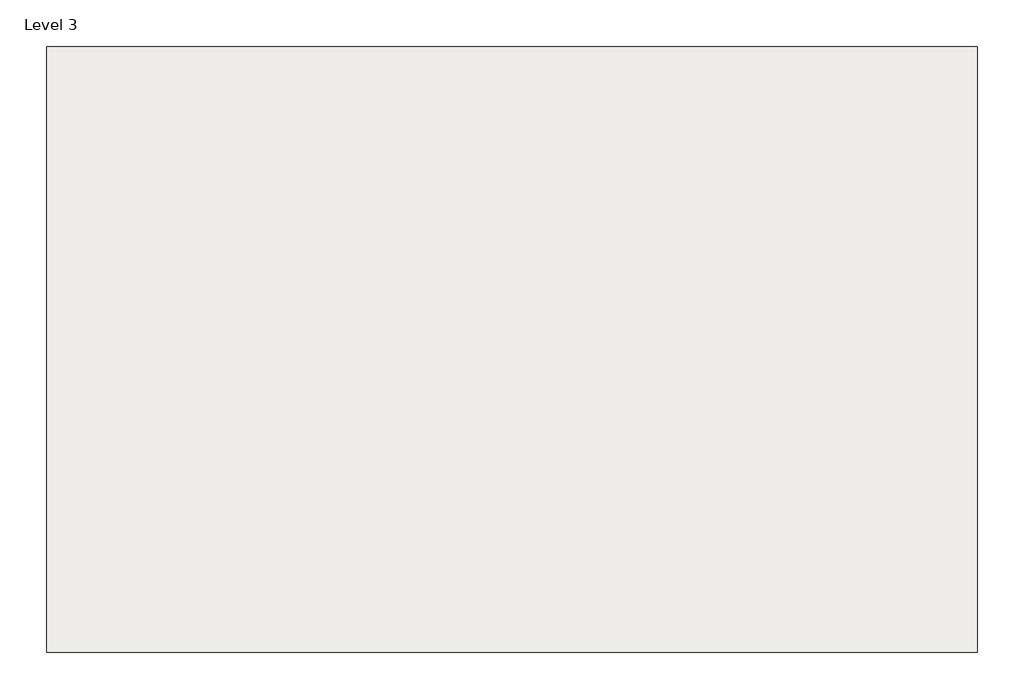
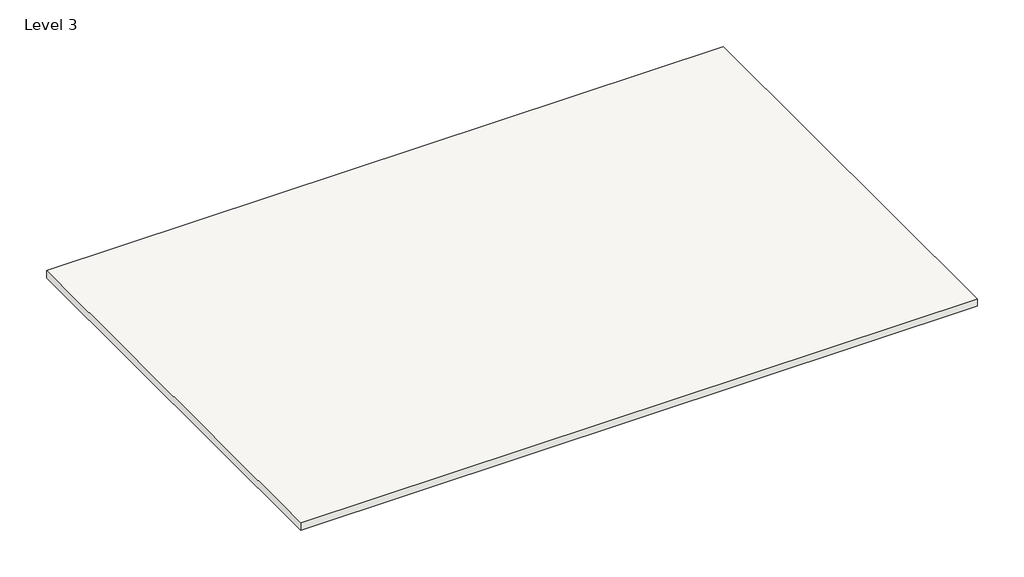
# One storey: 1 slab.
"""IFC4 building model written with IfcOpenShell, lengths in millimetres."""

from ifc_helpers import new_model, si_unit, frame, origin, place, context, project, spatial, polyline, outline, extrude, element, save

model = new_model("IFC4")

# Units and contexts
model_context = context("Model", 3, world=origin())
ifc_project = project(units=[si_unit("LENGTHUNIT", "METRE", prefix="MILLI")], contexts=[model_context])

# Site, building, storey
site = spatial("IfcSite", under=ifc_project)
building = spatial("IfcBuilding", under=site)
storey = spatial("IfcBuildingStorey", under=building, Name="Level 3", Elevation=6096.0)

# Slab
placement = place(None, origin())
element("IfcSlab", 1, ObjectType="6\"", at=placement, inside=storey, context=model_context, shape_type="SweptSolid", body=[
    extrude(outline(polyline([(-6312.7810046, 12034.9129661), (-6312.7810046, 3498.1962903), (-19437.2989325, 3498.1962903), (-19437.2989325, 12034.9129661), (-6312.7810046, 12034.9129661)])), frame((0.0, 0.0, 5943.6), z_axis=(0.0, 0.0, 1.0), x_axis=(1.0, 0.0, 0.0)), (0.0, 0.0, 1.0), 152.4),
])

save(model, "model.ifc")

# Revit data of these elements
# Type "6\""
#   Assembly Code = "B1010"
#   Function = 0
#   Layers, outside or top first: 0' - 6" no material (function 1)
# Element 1 (IfcSlab, "6\"")
#   Height Offset From Level = 0' - 0"
#   Phase Created = New Construction
#   Materials on its faces: "Default Floor"
# Materials
#   "Default Floor": colour RGB 128 128 128, transparency 0, Cost = 0
